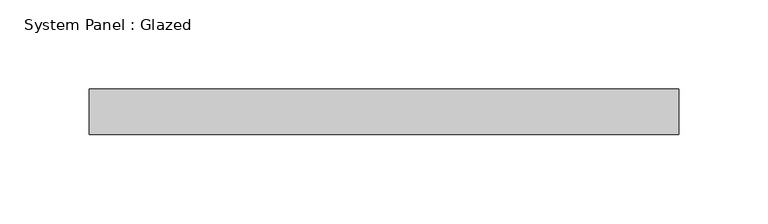
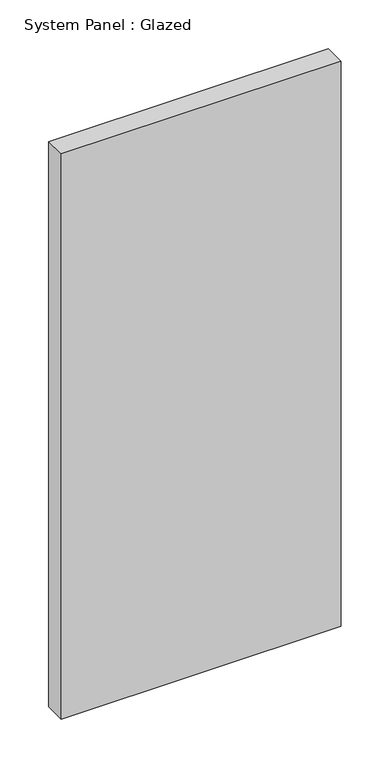
"""IFC4 building model written with IfcOpenShell, lengths in millimetres: plate geometry, System Panel : Glazed."""

from ifc_helpers import new_model, si_unit, origin, origin_with_axes, place, context, project, spatial, polyline, outline, extrude, source, transform, mapped, element, save


def system_panel_glazed_59fe5a42(model_context):
    return source(origin(), model_context, "Body", "SweptSolid", [
        extrude(outline(polyline([(165.1, 19.05), (-165.1, 19.05), (-165.1, 44.45), (165.1, 44.45), (165.1, 19.05)])), origin_with_axes(), (0.0, 0.0, 1.0), 705.0795173),
    ])


if __name__ == "__main__":
    model = new_model("IFC4")
    model_context = context("Model", 3, world=origin())
    ifc_project = project(units=[si_unit("LENGTHUNIT", "METRE", prefix="MILLI")], contexts=[model_context])
    site = spatial("IfcSite", under=ifc_project)
    building = spatial("IfcBuilding", under=site)
    placement = place(None, origin())
    system_panel_glazed_shape = system_panel_glazed_59fe5a42(model_context)
    element("IfcPlate", 1, ObjectType="System Panel : Glazed", at=placement, inside=building, context=model_context, shape_type="MappedRepresentation", body=[
        mapped(system_panel_glazed_shape, transform((0.0, 0.0, 0.0), x_axis=(1.0, 0.0, 0.0), y_axis=(0.0, 1.0, 0.0), z_axis=(0.0, 0.0, 1.0))),
    ])
    save(model, "model.ifc")

# Revit data of these elements
# Type "System Panel : Glazed"
#   Construction Type Id = "GSP4R"
#   Analytic Construction = "1/8 in Pilkington single glazing"
#   Visual Light Transmittance = 0.9
#   Solar Heat Gain Coefficient = 0.86
#   Heat Transfer Coefficient (U) = 1.18115 BTU/(h·ft²·°F)
#   Define Thermal Properties by = 1
# Element 1 (IfcPlate, "System Panel : Glazed")
#   Materials on its faces: "Glass"
# Materials
#   "Glass": class "Glass", colour RGB 0 128 192, transparency 0.75, Description = "Soda Lime Glass", Cost = 0
